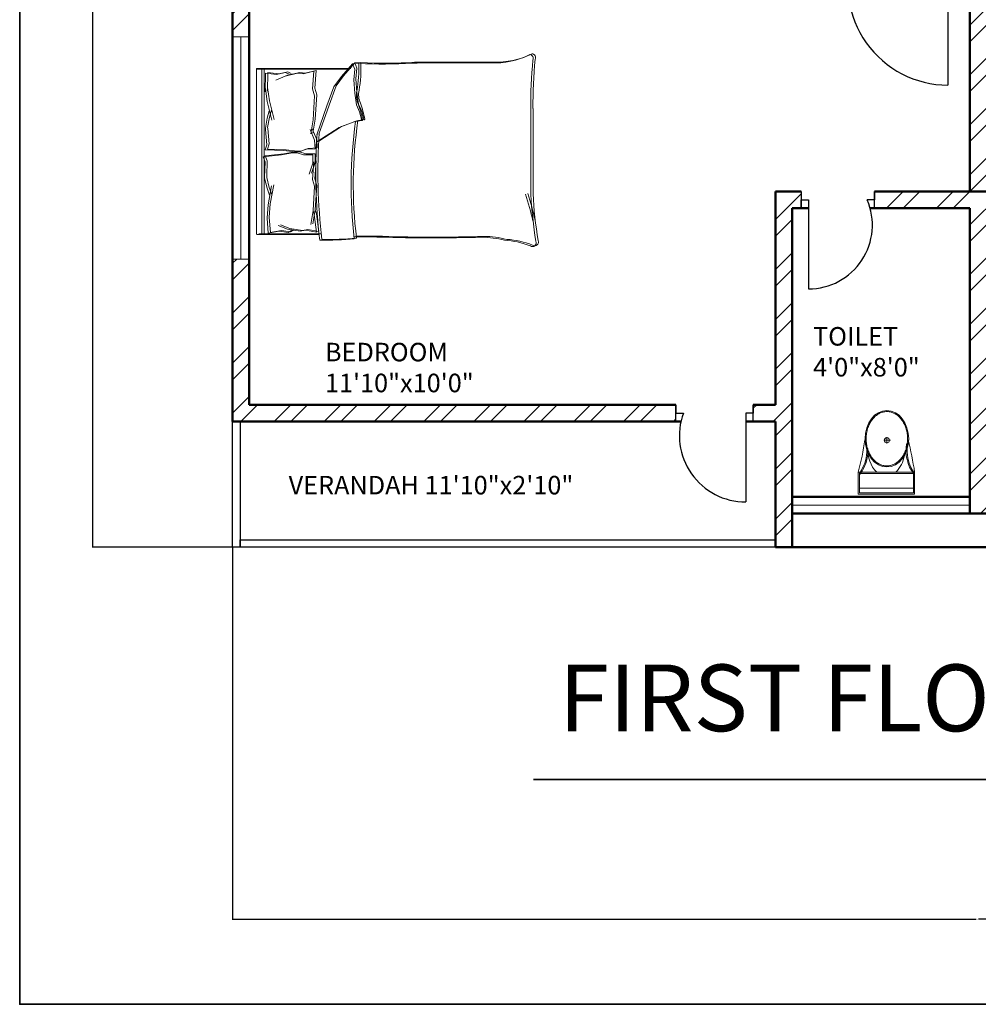
# Model space of a CAD drawing. Units: inches. Extents: x 2129 to 2642, y 1542 to 2414.
# Tile 1 of 9: x 2129 to 2388, y 1542 to 1808. Entities that reach past the tile are written whole.
import ezdxf

# ---------------------------------------------------------------- set-up
doc = ezdxf.new("R2010")
doc.units = ezdxf.units.IN
for name, color, linetype, lineweight in [('A-ANNO-DIMS', 2, 'Continuous', 18), ('A-ANNO-TITL', 7, 'Continuous', 35), ('A-ANNO-TTLB', 7, 'Continuous', 35), ('A-AREA-IDEN', 7, 'Continuous', 18), ('A-DOOR', 3, 'Continuous', 25), ('A-FLOR-FIXT', 9, 'Continuous', 18), ('A-FLOR-RAIL', 80, 'Continuous', 25), ('A-FURN', 8, 'Continuous', 18), ('A-GLAZ', 4, 'Continuous', 18), ('A-WALL', 7, 'Continuous', 50), ('A-WALL-PATT', 252, 'Continuous', 13)]:
    doc.layers.add(name, color=color, linetype=linetype, lineweight=lineweight)
doc.styles.get("Standard").update_dxf_attribs({"font": 'arial.ttf'})
doc.dimstyles.get("Standard").update_dxf_attribs({"dimtxt": 0.18, "dimasz": 0.18, "dimexe": 0.18, "dimexo": 0.0625, "dimgap": 0.09, "dimtad": 0, "dimtih": 1, "dimtoh": 1, "dimdec": 4, "dimzin": 0, "dimdsep": 46, "dimtxsty": 'Standard', "dimcen": 0.09, "dimadec": 0, "dimazin": 0, "dimtfac": 1, "dimtdec": 4, "dimtofl": 0, "dimtmove": 0, "dimatfit": 3, "dimfxl": 1, "dimtolj": 1, "dimtzin": 0, "dimarcsym": 0})

# ---------------------------------------------------------------- blocks, each defined once
blk = doc.blocks.new('A$C31115884')
for p, q in [((283.1, 497.7), (223.4, 497.7)), ((257.5, 466.4), (257.5, 523.2)), ((0, 200), (0, 0)), ((520, 200), (0, 200)), ((10, 190), (10, 10)), ((510, 190), (10, 190)), ((510, 10), (510, 190)), ((520, 0), (520, 200)), ((510, 54.5), (0, 54.5)), ((10, 10), (510, 10)), ((0, 0), (520, 0))]:
    blk.add_line(p, q)
blk.add_circle((255.6, 496.4), 23.6)
for centre, radius, start, end in [((2777.7, -204.6), 2807, 165.4549, 171.71327), ((-294.5, 403.3), 364.7, 324.20913, 9.34987), ((-294.5, 403.3), 374.7, 324.20913, 9.34987), ((805.8, 403.3), 364.7, 170.65013, 215.79087), ((3237, 905), 2807, 188.28673, 194.5451), ((139.5, 406.2), 293.5, 315.84364, 2.65635), ((805.8, 403.3), 374.7, 179.20365, 215.79087), ((383.6, 406.2), 293.5, 190.27735, 224.15636)]:
    blk.add_arc(centre, radius, start, end)
blk.add_ellipse((256.2, 509.9), major_axis=(0, -260.7), ratio=0.772727)
blk.add_open_spline([(256.2, 259.2), (263.1, 259.2), (270, 259.7), (287.8, 262.3), (298.7, 265.1), (319.9, 273.1), (330.2, 278.4), (350.1, 291.1), (359.7, 298.7), (377.7, 315.9), (386.2, 325.5), (401.7, 346.6), (408.8, 358.1), (421.3, 382.5), (426.8, 395.5), (435.9, 422.4), (439.5, 436.4), (444.8, 465.1), (446.5, 479.7), (447.9, 509.2), (447.6, 524), (445, 553.3), (442.7, 567.8), (436.3, 596), (432.1, 609.7), (421.9, 636), (416, 648.6), (402.5, 672.1), (395, 683), (378.6, 703), (369.8, 712.1), (351.1, 728), (341.3, 734.8), (320.9, 746.2), (310.4, 750.7), (288.9, 757.3), (278, 759.4), (256, 761), (245, 760.6), (223.1, 757.2), (212.3, 754.3), (191.1, 746.1), (180.8, 740.7), (160.9, 727.8), (151.4, 720.1), (133.5, 702.7), (125.1, 693), (109.6, 671.7), (102.6, 660.2), (90.2, 635.7), (84.9, 622.7), (76, 595.6), (72.4, 581.6), (67.2, 552.9), (65.6, 538.2), (64.4, 508.8), (64.8, 494), (67.5, 464.7), (69.9, 450.2), (76.6, 422), (80.8, 408.3), (91.1, 382.2), (97.2, 369.7), (110.8, 346.3), (118.4, 335.4), (134.8, 315.6), (143.7, 306.7), (162.4, 290.9), (172.3, 284.2), (192.8, 273), (203.3, 268.6), (224.8, 262.2), (235.8, 260.2), (249.9, 259.3), (253, 259.2), (256.2, 259.2)], degree=3, knots=[0, 0, 0, 0, 0.110105, 0.110105, 0.285049, 0.285049, 0.459994, 0.459994, 0.634938, 0.634938, 0.809882, 0.809882, 0.984827, 0.984827, 1.159771, 1.159771, 1.334715, 1.334715, 1.50966, 1.50966, 1.684604, 1.684604, 1.859549, 1.859549, 2.034493, 2.034493, 2.209437, 2.209437, 2.384382, 2.384382, 2.559326, 2.559326, 2.73427, 2.73427, 2.909215, 2.909215, 3.084159, 3.084159, 3.259103, 3.259103, 3.434048, 3.434048, 3.608992, 3.608992, 3.783936, 3.783936, 3.958881, 3.958881, 4.133825, 4.133825, 4.30877, 4.30877, 4.483714, 4.483714, 4.658658, 4.658658, 4.833603, 4.833603, 5.008547, 5.008547, 5.183491, 5.183491, 5.358436, 5.358436, 5.53338, 5.53338, 5.708324, 5.708324, 5.883269, 5.883269, 6.058213, 6.058213, 6.233158, 6.233158, 6.283185, 6.283185, 6.283185, 6.283185])
blk = doc.blocks.new('BED-DOUBLE')
for p, q in [((3.24, 59.14), (3.24, 76.05)), ((3.24, 74.61), (47.87, 74.61)), ((3.25, 59.14), (3.25, 76.05)), ((3.25, 74.61), (47.87, 74.61)), ((48.08, 76.05), (3.46, 76.05)), ((3.46, 58.54), (3.46, 75.45)), ((3.46, 58.54), (3.46, 75.45)), ((47.87, 76.05), (47.87, 51.2)), ((47.87, 76.05), (47.87, 51.2)), ((48.08, 76.05), (48.08, 75.45)), ((48.08, 75.45), (48.08, 50.6)), ((48.08, 75.45), (48.08, 50.6)), ((3.46, 74.02), (48.08, 74.02)), ((3.46, 74.02), (48.08, 74.02)), ((3.64, 72.93), (7.64, 73.24)), ((3.64, 72.93), (7.64, 73.24)), ((3.64, 72.95), (4.18, 69.98)), ((3.64, 72.95), (4.18, 69.98)), ((3.85, 72.33), (7.85, 72.64)), ((3.85, 72.33), (7.85, 72.64)), ((3.85, 72.35), (4.39, 69.38)), ((3.85, 72.35), (4.39, 69.38)), ((7.64, 73.24), (7.74, 73.22)), ((7.64, 73.24), (7.74, 73.22)), ((7.74, 73.22), (11.31, 72.95)), ((7.74, 73.22), (11.31, 72.95)), ((7.85, 72.64), (7.95, 72.62)), ((7.85, 72.64), (7.95, 72.62)), ((7.95, 72.62), (11.52, 72.35)), ((7.95, 72.62), (11.52, 72.35)), ((11.31, 72.95), (16.44, 72.01)), ((11.31, 72.95), (16.44, 72.01)), ((11.52, 72.35), (16.65, 71.41)), ((11.52, 72.35), (16.65, 71.41)), ((13.87, 72.55), (15.76, 73.22)), ((13.87, 72.55), (15.76, 73.22)), ((14.08, 71.95), (15.97, 72.62)), ((14.08, 71.95), (15.97, 72.62)), ((15.76, 73.22), (18.46, 73.9)), ((15.76, 73.22), (18.46, 73.9)), ((15.97, 72.62), (18.67, 73.3)), ((15.97, 72.62), (18.67, 73.3)), ((18.46, 73.9), (18.76, 73.9)), ((18.46, 73.9), (18.76, 73.9)), ((18.67, 73.3), (18.97, 73.3)), ((18.67, 73.3), (18.97, 73.3)), ((18.76, 73.9), (22.91, 73.76)), ((18.76, 73.9), (22.91, 73.76)), ((18.97, 73.3), (23.12, 73.16)), ((18.97, 73.3), (23.12, 73.16)), ((22.91, 73.76), (24.26, 74.3)), ((22.91, 73.76), (24.26, 74.3)), ((23.12, 73.16), (24.47, 73.7)), ((23.12, 73.16), (24.47, 73.7)), ((24.26, 74.3), (24.8, 69.31)), ((24.26, 74.3), (24.8, 69.31)), ((24.47, 73.7), (25.01, 68.71)), ((24.47, 73.7), (25.01, 68.71)), ((26.12, 73.72), (25.9, 68.7)), ((26.12, 73.72), (25.9, 68.7)), ((26.34, 73.12), (26.11, 68.1)), ((26.34, 73.12), (26.11, 68.1)), ((27.5, 73.27), (26.12, 73.72)), ((27.5, 73.27), (26.12, 73.72)), ((27.72, 72.67), (26.34, 73.12)), ((27.72, 72.67), (26.34, 73.12)), ((31.64, 73.66), (27.5, 73.27)), ((31.64, 73.66), (27.5, 73.27)), ((31.85, 73.06), (27.72, 72.67)), ((31.85, 73.06), (27.72, 72.67)), ((31.94, 73.68), (31.64, 73.66)), ((31.94, 73.68), (31.64, 73.66)), ((32.15, 73.08), (31.85, 73.06)), ((32.15, 73.08), (31.85, 73.06)), ((34.68, 73.17), (31.94, 73.68)), ((34.67, 73.17), (31.94, 73.68)), ((34.89, 72.58), (32.15, 73.08)), ((34.89, 72.58), (32.15, 73.08)), ((39.14, 73.18), (34.08, 71.92)), ((39.14, 73.18), (34.08, 71.92)), ((39.35, 72.58), (34.29, 71.32)), ((39.35, 72.58), (34.29, 71.32)), ((36.6, 72.62), (34.67, 73.17)), ((36.6, 72.62), (34.68, 73.17)), ((36.82, 72.02), (34.89, 72.58)), ((36.82, 72.02), (34.89, 72.58)), ((42.68, 73.67), (39.14, 73.18)), ((42.68, 73.67), (39.14, 73.18)), ((42.9, 73.08), (39.35, 72.58)), ((42.9, 73.08), (39.35, 72.58)), ((46.79, 73.66), (41.75, 73.75)), ((41.75, 73.75), (42.68, 73.67)), ((46.79, 73.66), (41.75, 73.75)), ((41.75, 73.75), (42.68, 73.67)), ((47.01, 73.06), (41.96, 73.15)), ((41.96, 73.15), (42.9, 73.08)), ((47.01, 73.06), (41.96, 73.15)), ((41.96, 73.15), (42.9, 73.08)), ((46.79, 73.66), (46.44, 70.66)), ((46.79, 73.66), (46.44, 70.66)), ((47.01, 73.06), (46.65, 70.06)), ((47.01, 73.06), (46.65, 70.06)), ((4.18, 69.98), (3.77, 67.55)), ((4.18, 69.98), (3.77, 67.55)), ((4.39, 69.38), (3.98, 66.95)), ((4.39, 69.38), (3.99, 66.95)), ((4.72, 67.69), (5.66, 70.25)), ((4.72, 67.69), (5.66, 70.25)), ((4.93, 67.09), (5.87, 69.65)), ((4.93, 67.09), (5.87, 69.65)), ((24.8, 69.31), (25.34, 66.34)), ((24.8, 69.31), (25.34, 66.34)), ((46.04, 68.34), (44.94, 70.84)), ((46.04, 68.34), (44.94, 70.84)), ((46.26, 67.74), (45.15, 70.24)), ((46.26, 67.74), (45.15, 70.24)), ((46.44, 70.66), (46.99, 68.26)), ((46.44, 70.66), (46.99, 68.26)), ((46.65, 70.06), (47.21, 67.66)), ((46.65, 70.06), (47.21, 67.66)), ((3.77, 67.55), (4.31, 66.61)), ((3.77, 67.55), (4.31, 66.61)), ((3.98, 66.95), (4.52, 66.01)), ((3.99, 66.95), (4.53, 66.01)), ((4.18, 64.31), (4.72, 67.69)), ((4.18, 64.31), (4.72, 67.69)), ((4.39, 63.71), (4.93, 67.09)), ((4.39, 63.71), (4.93, 67.09)), ((25.01, 68.71), (25.55, 65.74)), ((25.01, 68.71), (25.55, 65.74)), ((25.9, 68.7), (25.54, 65.7)), ((25.9, 68.7), (25.54, 65.7)), ((26.11, 68.1), (25.76, 65.11)), ((26.11, 68.1), (25.76, 65.11)), ((46.79, 65), (46.04, 68.34)), ((46.79, 65), (46.04, 68.34)), ((47.01, 64.41), (46.26, 67.74)), ((47.01, 64.41), (46.26, 67.74)), ((46.99, 68.26), (46.51, 67.28)), ((46.99, 68.26), (46.51, 67.28)), ((47.21, 67.66), (46.73, 66.69)), ((47.21, 67.66), (46.73, 66.69)), ((4.45, 62.82), (4.18, 64.31)), ((4.45, 62.82), (4.18, 64.31)), ((25.34, 65.12), (24.8, 63.36)), ((25.34, 65.12), (24.8, 63.36)), ((25.55, 64.52), (25.01, 62.77)), ((25.55, 64.52), (25.01, 62.77)), ((25.34, 66.34), (25.34, 65.12)), ((25.34, 66.34), (25.34, 65.12)), ((25.54, 65.7), (25.62, 64.49)), ((25.54, 65.7), (25.62, 64.49)), ((25.55, 65.74), (25.55, 64.52)), ((25.55, 65.74), (25.55, 64.52)), ((25.62, 64.49), (26.27, 62.77)), ((25.62, 64.49), (26.27, 62.77)), ((25.76, 65.11), (25.83, 63.89)), ((25.76, 65.11), (25.83, 63.89)), ((25.83, 63.89), (26.48, 62.18)), ((25.83, 63.89), (26.48, 62.18)), ((46.62, 63.5), (46.79, 65)), ((46.62, 63.5), (46.79, 65)), ((46.83, 62.91), (47.01, 64.41)), ((46.83, 62.91), (47.01, 64.41)), ((3.91, 59.85), (4.45, 62.82)), ((3.91, 59.85), (4.45, 62.82)), ((4.12, 59.26), (4.66, 62.23)), ((4.12, 59.26), (4.66, 62.23)), ((4.66, 62.23), (4.39, 63.71)), ((4.66, 62.23), (4.39, 63.71)), ((5.96, 61.45), (9.72, 60.83)), ((5.96, 61.45), (9.72, 60.83)), ((22.51, 60.86), (19.57, 61.88)), ((22.51, 60.86), (19.57, 61.88)), ((22.72, 60.26), (19.78, 61.28)), ((22.72, 60.26), (19.78, 61.28)), ((24.8, 63.36), (24.8, 60.86)), ((24.8, 63.36), (24.8, 60.86)), ((25.01, 62.77), (25.01, 60.26)), ((25.01, 62.77), (25.01, 60.26)), ((26.27, 62.77), (26.42, 60.27)), ((26.27, 62.77), (26.42, 60.27)), ((26.48, 62.18), (26.64, 59.68)), ((26.48, 62.18), (26.64, 59.68)), ((28.71, 60.42), (31.58, 61.62)), ((28.71, 60.42), (31.58, 61.62)), ((30.41, 61.45), (34.17, 60.83)), ((30.41, 61.45), (34.17, 60.83)), ((47.34, 60.57), (46.62, 63.5)), ((47.34, 60.57), (46.62, 63.5)), ((47.55, 59.98), (46.83, 62.91)), ((47.55, 59.98), (46.83, 62.91)), ((8.67, 60.53), (3.91, 59.85)), ((8.67, 60.53), (3.91, 59.85)), ((8.88, 59.93), (4.12, 59.26)), ((8.88, 59.93), (4.12, 59.26)), ((6.17, 60.86), (9.94, 60.23)), ((6.17, 60.86), (9.94, 60.23)), ((9.72, 60.83), (8.67, 60.53)), ((9.72, 60.83), (8.67, 60.53)), ((9.94, 60.23), (8.88, 59.93)), ((9.94, 60.23), (8.88, 59.93)), ((9.72, 60.83), (16.27, 60.43)), ((9.72, 60.83), (16.27, 60.43)), ((9.94, 60.23), (16.48, 59.83)), ((9.94, 60.23), (16.48, 59.83)), ((16.27, 60.43), (18.1, 60.95)), ((16.27, 60.43), (18.1, 60.95)), ((16.48, 59.83), (18.31, 60.35)), ((16.48, 59.83), (18.31, 60.35)), ((18.1, 60.95), (22.89, 60.57)), ((18.1, 60.95), (22.89, 60.57)), ((18.31, 60.35), (23.11, 59.98)), ((18.31, 60.35), (23.1, 59.98)), ((24.8, 60.86), (22.51, 60.86)), ((24.8, 60.86), (22.51, 60.86)), ((25.01, 60.26), (22.72, 60.26)), ((25.01, 60.26), (22.72, 60.26)), ((26.42, 60.27), (28.71, 60.42)), ((26.42, 60.27), (28.71, 60.42)), ((26.64, 59.68), (28.93, 59.82)), ((26.64, 59.68), (28.93, 59.82)), ((28.25, 59.82), (32.17, 53.75)), ((28.25, 59.82), (32.17, 53.75)), ((28.47, 59.22), (32.38, 53.16)), ((28.47, 59.22), (32.38, 53.16)), ((28.93, 59.82), (31.79, 61.02)), ((28.93, 59.82), (31.79, 61.02)), ((37.95, 57.08), (30.17, 59.82)), ((37.95, 57.08), (30.17, 59.82)), ((38.16, 56.48), (30.38, 59.22)), ((38.16, 56.48), (30.38, 59.22)), ((30.62, 60.86), (34.39, 60.23)), ((30.62, 60.86), (34.38, 60.23)), ((34.17, 60.83), (40.72, 60.43)), ((34.17, 60.83), (40.72, 60.43)), ((34.38, 60.23), (40.93, 59.83)), ((34.39, 60.23), (40.93, 59.83)), ((40.72, 60.43), (42.55, 60.95)), ((40.72, 60.43), (42.55, 60.95)), ((40.93, 59.83), (42.76, 60.35)), ((40.93, 59.83), (42.76, 60.35)), ((42.55, 60.95), (47.34, 60.57)), ((42.55, 60.95), (47.34, 60.57)), ((42.76, 60.35), (47.55, 59.98)), ((42.76, 60.35), (47.55, 59.98)), ((43.16, 55.2), (37.95, 57.08)), ((43.16, 55.2), (37.95, 57.08)), ((43.37, 54.6), (38.16, 56.48)), ((43.37, 54.6), (38.16, 56.48)), ((32.17, 53.75), (33.76, 49.56)), ((32.17, 53.75), (33.76, 49.56)), ((32.38, 53.16), (33.97, 48.96)), ((32.38, 53.16), (33.97, 48.96)), ((45.91, 53.17), (43.16, 55.2)), ((45.91, 53.17), (43.16, 55.2)), ((46.12, 52.58), (43.37, 54.6)), ((46.12, 52.58), (43.37, 54.6)), ((49.37, 50.14), (45.91, 53.17)), ((49.36, 50.14), (45.91, 53.17)), ((49.58, 49.54), (46.12, 52.58)), ((49.58, 49.54), (46.12, 52.58)), ((33.76, 49.56), (34.05, 47.68)), ((33.76, 49.56), (34.05, 47.68)), ((33.97, 48.96), (34.26, 47.09)), ((33.97, 48.96), (34.26, 47.09)), ((34.05, 47.68), (36.36, 48.26)), ((34.05, 47.68), (36.36, 48.26)), ((36.36, 48.26), (38.24, 49.13)), ((36.36, 48.26), (38.24, 49.13)), ((36.57, 47.66), (38.45, 48.53)), ((36.57, 47.66), (38.45, 48.53)), ((38.24, 49.13), (41.42, 49.56)), ((38.24, 49.13), (41.42, 49.56)), ((38.45, 48.53), (41.64, 48.96)), ((38.45, 48.53), (41.64, 48.96)), ((41.42, 49.56), (45.04, 49.85)), ((41.42, 49.56), (45.04, 49.85)), ((41.64, 48.96), (45.25, 49.25)), ((41.64, 48.96), (45.25, 49.25)), ((45.04, 49.85), (47.93, 49.56)), ((45.04, 49.85), (47.93, 49.56)), ((45.25, 49.25), (48.14, 48.96)), ((45.25, 49.25), (48.14, 48.96)), ((47.93, 49.56), (49.37, 50.14)), ((47.93, 49.56), (49.36, 50.14)), ((48.14, 48.96), (49.58, 49.54)), ((48.14, 48.96), (49.58, 49.54)), ((49.44, 48.51), (49.36, 50.14, 3.61)), ((49.44, 48.51), (49.37, 50.14, 3.61)), ((49.65, 47.91), (49.58, 49.54, 3.61)), ((49.65, 47.91), (49.58, 49.54, 3.61)), ((34.26, 47.09), (36.57, 47.66)), ((34.26, 47.09), (36.57, 47.66)), ((14.07, 2.05), (37.05, 2.05)), ((14.07, 2.05), (37.05, 2.05)), ((14.28, 1.46), (37.26, 1.46)), ((14.28, 1.46), (37.26, 1.46))]:
    blk.add_line(p, q)
for centre, radius, start, end in [((79.52, 57.28), 77.79, 178.7218, 185.604), ((79.52, 57.28), 77.79, 178.7218, 185.604), ((19.94, -93.94), 154.04, 86.0865, 96.7821), ((19.94, -93.94), 154.04, 86.0865, 96.7821), ((20.16, -94.54), 154.04, 86.0865, 96.7821), ((20.16, -94.54), 154.04, 86.0865, 96.7821), ((79.73, 56.69), 77.79, 178.7218, 185.604), ((79.73, 56.69), 77.79, 178.7218, 185.604), ((16.58, -69.91), 120.47, 81.7845, 96.9006), ((16.58, -69.91), 120.47, 81.7845, 96.9006), ((16.79, -70.51), 120.47, 81.7845, 96.9006), ((16.79, -70.51), 120.47, 81.7845, 96.9006), ((-156.22, 46.94), 158.84, 358.4762, 1.0082), ((-156.22, 46.94), 158.84, 358.4762, 1.0082), ((-156.01, 46.34), 158.84, 358.4762, 1.0082), ((-156.01, 46.34), 158.84, 358.4762, 1.0082), ((29.09, 74.66), 27.69, 280.6617, 289.8806), ((29.09, 74.66), 27.69, 280.6617, 289.8806), ((29.3, 74.07), 27.69, 280.6617, 289.8806), ((29.3, 74.07), 27.69, 280.6617, 289.8806), ((40.85, 43.3), 5.81, 78.6608, 113.7384), ((40.85, 43.3), 5.81, 78.6608, 113.7384), ((41.06, 42.71), 5.81, 78.6608, 113.7384), ((41.06, 42.71), 5.81, 78.6608, 113.7384), ((47.93, 82.26), 33.79, 259.8763, 272.5657), ((47.93, 82.26), 33.79, 259.8763, 272.5657), ((48.14, 81.67), 33.79, 259.8763, 272.5657), ((48.14, 81.67), 33.79, 259.8763, 272.5657), ((170.19, 42.14), 120.92, 176.9791, 183.8365), ((170.19, 42.14), 120.92, 176.9791, 183.8365), ((170.4, 41.54), 120.92, 176.9791, 183.8365), ((170.4, 41.54), 120.92, 176.9791, 183.8365), ((34.21, 47.62), 0.172, 160.2464, 271.1377), ((34.21, 47.62), 0.172, 160.2464, 271.1377), ((34.42, 47.03), 0.172, 160.2464, 271.1377), ((34.42, 47.03), 0.172, 160.2464, 271.1377), ((452.7, 28.79), 450.36, 178.2277, 181.7185), ((452.7, 28.79), 450.36, 178.2277, 181.7185), ((452.91, 28.19), 450.36, 178.2277, 181.7185), ((452.91, 28.19), 450.36, 178.2277, 181.7185), ((-4210.02, 12.72), 4259.62, 0.00217, 0.28689), ((-4210.02, 12.72), 4259.62, 0.00217, 0.28689), ((-4209.81, 12.12), 4259.62, 0.00217, 0.28689), ((-4209.81, 12.12), 4259.62, 0.00217, 0.28689), ((-25.12, 15.81), 27.67, 346.0648, 358.9113), ((-25.12, 15.81), 27.67, 346.0648, 358.9113), ((-24.9, 15.21), 27.67, 346.0648, 358.9113), ((-24.9, 15.21), 27.67, 346.0648, 358.9113), ((71.11, 11.93), 21.54, 177.4714, 206.4681), ((71.11, 11.93), 21.54, 177.4714, 206.4681), ((71.33, 11.33), 21.54, 177.4714, 206.4681), ((71.32, 11.33), 21.54, 177.4714, 206.4681), ((-20.22, 10.43), 22, 337.9751, 356.652), ((-20.22, 10.43), 22, 337.9751, 356.652), ((-20.01, 9.83), 22, 337.9751, 356.652), ((-20.01, 9.83), 22, 337.9751, 356.652), ((-16.08, 98.19), 99.41, 283.3832, 287.7053), ((-16.08, 98.19), 99.41, 283.3832, 287.7053), ((-15.87, 97.59), 99.41, 283.3832, 287.7053), ((-15.87, 97.59), 99.41, 283.3832, 287.7053), ((1.02, 1.61), 1.02, 146.1736, 293.4781), ((1.02, 1.61), 1.02, 146.1736, 293.4781), ((1.23, 1.01), 1.02, 146.1736, 293.4781), ((1.23, 1.01), 1.02, 146.1736, 293.4781), ((20.01, -111.48), 113.69, 92.9958, 99.4091), ((20.01, -111.48), 113.69, 92.9958, 99.4091), ((20.22, -112.08), 113.69, 92.9958, 99.4091), ((20.22, -112.08), 113.69, 92.9958, 99.4091), ((38.43, -122.17), 124.23, 84.4998, 90.6351), ((38.43, -122.17), 124.23, 84.4998, 90.6351), ((38.64, -122.76), 124.23, 84.4998, 90.6351), ((38.64, -122.76), 124.23, 84.4998, 90.6351), ((50.81, 2.4), 1.03, 242.6588, 356.02), ((50.81, 2.4), 1.03, 242.6588, 356.02), ((51.02, 1.81), 1.03, 242.6588, 356.02), ((51.02, 1.81), 1.03, 242.6588, 356.02)]:
    blk.add_arc(centre, radius, start, end)
blk = doc.blocks.new('WIN-60-B')
for p, q in [((4.5, 60), (0, 60)), ((0, 60), (2.25, 60)), ((2.25, 60), (2.25, 0)), ((2.25, 0), (0, 0)), ((0, 0), (4.5, 0))]:
    blk.add_line(p, q)
blk = doc.blocks.new('*D34')
at = {"layer": 'A-ANNO-DIMS', "color": 0, "lineweight": -2, "transparency": 16777216}
for p, q in [((2186.9, 1665.66), (2186.9, 1565.16)), ((2588.9, 1665.66), (2588.9, 1565.16)), ((2187.08, 1565.34), (2387.61, 1565.34)), ((2588.72, 1565.34), (2388.2, 1565.34))]:
    blk.add_line(p, q, dxfattribs=at)
at = {"layer": 'A-ANNO-DIMS', "color": 0, "transparency": 16777216}
for points in [[(2187.08, 1565.37), (2187.08, 1565.31), (2186.9, 1565.34)], [(2588.72, 1565.37), (2588.72, 1565.31), (2588.9, 1565.34)]]:
    blk.add_solid(points, dxfattribs=at)
at = {"layer": 'Defpoints', "color": 0, "transparency": 16777216}
for p in [(2186.9, 1665.72), (2588.9, 1665.72), (2588.9, 1565.34)]:
    blk.add_point(p, dxfattribs=at)
at = {"layer": 'A-ANNO-DIMS', "color": 0, "transparency": 16777216, "insert": (2387.9, 1565.34), "char_height": 0.18, "attachment_point": 5}
blk.add_mtext('\\A1;402', dxfattribs=at)
blk = doc.blocks.new('*D35')
at = {"layer": 'A-ANNO-DIMS', "color": 0, "lineweight": -2, "transparency": 16777216}
for p, q in [((2186.84, 2340.22), (2148.97, 2340.22)), ((2149.15, 2340.04), (2149.15, 2003.15)), ((2149.15, 1665.9), (2149.15, 2002.79)), ((2186.84, 1665.72), (2148.97, 1665.72))]:
    blk.add_line(p, q, dxfattribs=at)
at = {"layer": 'A-ANNO-DIMS', "color": 0, "transparency": 16777216}
for points in [[(2149.12, 2340.04), (2149.18, 2340.04), (2149.15, 2340.22)], [(2149.12, 1665.9), (2149.18, 1665.9), (2149.15, 1665.72)]]:
    blk.add_solid(points, dxfattribs=at)
at = {"layer": 'Defpoints', "color": 0, "transparency": 16777216}
for p in [(2149.15, 2340.22), (2186.9, 2340.22), (2186.9, 1665.72)]:
    blk.add_point(p, dxfattribs=at)
at = {"layer": 'A-ANNO-DIMS', "color": 0, "transparency": 16777216, "insert": (2149.15, 2002.97), "char_height": 0.18, "attachment_point": 5}
blk.add_mtext('\\A1;674.5', dxfattribs=at)

msp = doc.modelspace()

# ---------------------------------------------------------------- hatches: boundary and pattern name
at = {"layer": 'A-WALL-PATT'}
h = msp.add_hatch(dxfattribs=at)
h.set_pattern_fill('ANSI32', color=256)
h.paths.add_polyline_path([(2306.2606, 2305.9717), (2306.2606, 2308.2217), (2276.3515, 2308.2217), (2276.3515, 2303.7217), (2306.2606, 2303.7217)])
h.paths.add_polyline_path([(2216.3515, 2305.9717), (2216.3515, 2308.2217), (2186.9043, 2308.2217), (2186.9043, 2278.1696), (2191.4043, 2278.1696), (2191.4043, 2303.7217), (2216.3515, 2303.7217)])
h.paths.add_polyline_path([(2339.9043, 2335.7217), (2362.1938, 2335.7217), (2362.1938, 2340.2217), (2335.4043, 2340.2217), (2335.4043, 2308.2217), (2329.3487, 2308.2217), (2329.3487, 2305.9717), (2329.3487, 2303.7217), (2335.4043, 2303.7217), (2335.4043, 2186.7217), (2329.4345, 2186.7217), (2329.4345, 2182.2217), (2335.4043, 2182.2217), (2335.4043, 2174.7178), (2339.9043, 2174.7178), (2339.9043, 2182.2217), (2339.9043, 2303.7217)])
h.paths.add_polyline_path([(2440.4043, 2340.2217), (2411.654, 2340.2217), (2411.654, 2335.7217), (2435.9043, 2335.7217), (2435.9043, 2303.7217), (2435.9043, 2182.2217), (2435.9043, 2174.1935), (2438.1543, 2174.1935), (2440.4043, 2174.1935), (2440.4043, 2182.2217), (2444.653, 2182.2217), (2444.653, 2184.4717), (2444.653, 2186.7217), (2440.4043, 2186.7217), (2440.4043, 2303.7217), (2445.8547, 2303.7217), (2445.8547, 2308.2217), (2440.4043, 2308.2217)])
h.paths.add_polyline_path([(2498.2381, 2308.2217), (2470.3901, 2308.2217), (2470.3901, 2303.7217), (2498.2381, 2303.7217), (2498.2381, 2305.9717)])
h.paths.add_polyline_path([(2588.9043, 2308.2217), (2586.9043, 2308.2217), (2558.2381, 2308.2217), (2558.2381, 2303.7217), (2584.4043, 2303.7217), (2584.4043, 2279.1087), (2588.9043, 2279.1087)])
h.paths.add_polyline_path([(2588.9043, 2219.1087), (2584.4043, 2219.1087), (2584.4043, 2186.7217), (2478.0667, 2186.7217), (2478.0667, 2182.2217), (2584.4043, 2182.2217), (2584.4043, 2157.7883), (2588.9043, 2157.7883)])
h.paths.add_polyline_path([(2588.9043, 2097.7883), (2584.6063, 2097.7883), (2584.6063, 2075.5462, -0.09241561), (2584.4043, 2074.4627), (2584.4043, 2064.2217), (2495.9043, 2064.2217), (2495.9043, 2040.4611), (2500.4043, 2040.4611), (2500.4043, 2059.7217), (2584.4043, 2059.7217), (2584.4043, 2052.2164), (2588.9043, 2052.2164)])
h.paths.add_polyline_path([(2588.9043, 2028.2164), (2584.4043, 2028.2164), (2584.4043, 2011.7217), (2500.4043, 2011.7217), (2500.4043, 2015.243), (2498.1543, 2015.243), (2495.9043, 2015.243), (2495.9043, 2007.2217), (2495.9043, 2003.7597), (2500.4043, 2003.7597), (2500.4043, 2007.2217), (2584.4043, 2007.2217), (2584.4043, 1992.1997), (2588.9043, 1992.1997)])
h.paths.add_polyline_path([(2588.9043, 1956.1997), (2584.4043, 1956.1997), (2584.4043, 1941.2217), (2500.4043, 1941.2217), (2500.4043, 1985.1493), (2498.1543, 1985.1493), (2495.9043, 1985.1493), (2495.9043, 1941.2217), (2435.9043, 1941.2217), (2435.9043, 1930.3963), (2440.4043, 1930.3963), (2440.4043, 1936.7217), (2584.4043, 1936.7217), (2584.4043, 1909.8406), (2588.9043, 1909.8406)])
h.paths.add_polyline_path([(2588.9043, 1849.8406), (2584.4043, 1849.8406), (2584.4043, 1801.3526), (2588.9043, 1801.3526)])
h.paths.add_polyline_path([(2584.4043, 1828.7217), (2495.9043, 1828.7217), (2440.4043, 1828.7217), (2440.4043, 1905.2159), (2438.1543, 1905.2159), (2435.9043, 1905.2159), (2435.9043, 1828.7217), (2428.9101, 1828.7217), (2428.9101, 1824.2217), (2584.4043, 1824.2217)])
h.paths.add_polyline_path([(2588.9043, 1741.3526), (2584.4043, 1741.3526), (2584.4043, 1704.2217), (2468.3173, 1704.2217), (2468.3173, 1701.9717), (2468.3173, 1699.7217), (2588.9043, 1699.7217)])
h.paths.add_polyline_path([(2442.4043, 1761.7217), (2435.0216, 1761.7217), (2435.0216, 1757.2217), (2437.9043, 1757.2217), (2437.9043, 1665.7217), (2442.4043, 1665.7217), (2442.4043, 1667.7217), (2442.4043, 1699.7217), (2446.6907, 1699.7217), (2446.6907, 1701.9717), (2446.6907, 1704.2217), (2442.4043, 1704.2217)])
h.paths.add_polyline_path([(2390.4043, 1757.2217), (2410.8996, 1757.2217), (2410.8996, 1761.7217), (2360.1741, 1761.7217), (2360.1741, 1759.4717), (2360.1741, 1757.2217), (2385.9043, 1757.2217), (2385.9043, 1674.8326), (2390.4043, 1674.8326)])
h.paths.add_polyline_path([(2337.9043, 1757.2217), (2340.3592, 1757.2217), (2340.3592, 1759.4717), (2340.3592, 1761.7217), (2333.4043, 1761.7217), (2333.4043, 1704.2217), (2327.381, 1704.2217), (2327.381, 1701.9717), (2327.381, 1699.7217), (2333.4043, 1699.7217), (2333.4043, 1665.7217), (2337.9043, 1665.7217)])
h.paths.add_polyline_path([(2191.4043, 1743.4804), (2186.9043, 1743.4804), (2186.9043, 1699.7217), (2188.9043, 1699.7217), (2191.4043, 1699.7217), (2306.5617, 1699.7217), (2306.5617, 1704.2217), (2191.4043, 1704.2217)])
h.paths.add_polyline_path([(2191.4043, 1859.8992), (2186.9043, 1859.8992), (2186.9043, 1803.4804), (2189.1543, 1803.4804), (2191.4043, 1803.4804)])
h.paths.add_polyline_path([(2352.5445, 1828.7217), (2191.4043, 1828.7217), (2191.4043, 1824.2217), (2333.4043, 1824.2217), (2352.5445, 1824.2217), (2352.5445, 1826.4717)])
h.paths.add_polyline_path([(2390.4043, 2085.328), (2385.9043, 2085.328), (2385.9043, 1828.7217), (2381.9668, 1828.7217), (2381.9668, 1826.4717), (2381.9668, 1824.2217), (2385.9043, 1824.2217), (2385.9043, 1761.7217), (2390.4043, 1761.7217), (2390.4043, 1824.2217), (2394.1868, 1824.2217), (2394.1868, 1827.6339), (2394.1868, 1828.7217), (2390.4043, 1828.7217)])
h.paths.add_polyline_path([(2339.9043, 1941.2217), (2335.4043, 1941.2217), (2279.9043, 1941.2217), (2279.9043, 1981.3432), (2277.6543, 1981.3432), (2275.4043, 1981.3432), (2275.4043, 1941.2217), (2191.4043, 1941.2217), (2191.4043, 1958.1079), (2186.9043, 1958.1079), (2186.9043, 1919.8992), (2189.1543, 1919.8992), (2191.4043, 1919.8992), (2191.4043, 1936.7217), (2279.9043, 1936.7217), (2335.4043, 1936.7217), (2335.4043, 1931.1382), (2339.9043, 1931.1382)])
h.paths.add_polyline_path([(2339.9043, 1902.7544), (2337.6543, 1902.7544), (2335.4043, 1902.7544), (2335.4043, 1828.7217), (2339.9043, 1828.7217)])
h.paths.add_polyline_path([(2279.9043, 2015.263), (2277.6543, 2015.263), (2275.4043, 2015.263), (2275.4043, 2011.7217), (2191.4043, 2011.7217), (2191.4043, 2026.6781), (2186.9043, 2026.6781), (2186.9043, 1994.1079), (2189.1543, 1994.1079), (2191.4043, 1994.1079), (2191.4043, 2007.2217), (2275.4043, 2007.2217), (2275.4043, 2003.2288), (2279.9043, 2003.2288), (2279.9043, 2007.2217)])
h.paths.add_polyline_path([(2296.0216, 2186.7217), (2191.4043, 2186.7217), (2191.4043, 2218.1696), (2186.9043, 2218.1696), (2186.9043, 2158.4509), (2191.4043, 2158.4509), (2191.4043, 2182.2217), (2296.0216, 2182.2217), (2296.0216, 2184.4717)])
h.paths.add_polyline_path([(2191.4043, 2098.4509), (2189.1543, 2098.4509), (2186.9043, 2098.4509), (2186.9043, 2050.6781), (2189.0487, 2050.6781), (2191.4043, 2050.6781), (2191.4043, 2059.7217), (2275.4043, 2059.7217), (2275.4043, 2038.4133), (2279.9043, 2038.4133), (2279.9043, 2064.2217), (2191.4043, 2064.2217)])
h.paths.add_polyline_path([(2268.3923, 1605.9386), (2516.3159, 1605.9386), (2516.3159, 1643.0314), (2268.3923, 1643.0314)], flags=9)
h.paths.add_polyline_path([(2399.6079, 1710.4489), (2428.8405, 1710.4489), (2428.8405, 1729.1062), (2399.6079, 1729.1062)], flags=9)
h.paths.add_polyline_path([(2342.1483, 1708.9956), (2371.3809, 1708.9956), (2371.3809, 1727.653), (2342.1483, 1727.653)], flags=9)
h.paths.add_polyline_path([(2200.7404, 1677.2519), (2282.3059, 1677.2519), (2282.3059, 1687.5555), (2200.7404, 1687.5555)], flags=9)
h.paths.add_polyline_path([(2209.8153, 1704.7448), (2250.627, 1704.7448), (2250.627, 1723.4021), (2209.8153, 1723.4021)], flags=25)
h.paths.add_polyline_path([(2213.9996, 1911.284), (2252.84, 1911.284), (2252.84, 1929.9413), (2213.9996, 1929.9413)], flags=9)
h.paths.add_polyline_path([(2210.8865, 1962.0987), (2244.0447, 1962.0987), (2244.0447, 1980.7561), (2210.8865, 1980.7561)], flags=25)
h.paths.add_polyline_path([(2219.0745, 2037.6131), (2248.2321, 2037.6131), (2248.2321, 2056.2705), (2219.0745, 2056.2705)], flags=9)
h.paths.add_polyline_path([(2379.9702, 2099.0686), (2409.3767, 2099.0686), (2409.3767, 2117.7259), (2379.9702, 2117.7259)], flags=9)
h.paths.add_polyline_path([(2375.9312, 2160.3752), (2405.3173, 2160.3752), (2405.3173, 2179.0325), (2375.9312, 2179.0325)], flags=9)
h.paths.add_polyline_path([(2269.5058, 2112.1824), (2310.3175, 2112.1824), (2310.3175, 2130.8397), (2269.5058, 2130.8397)], flags=9)
h.paths.add_polyline_path([(2209.6567, 2193.667), (2248.4971, 2193.667), (2248.4971, 2212.3243), (2209.6567, 2212.3243)], flags=25)
h.paths.add_polyline_path([(2491.6289, 1675.447), (2573.1944, 1675.447), (2573.1944, 1685.7506), (2491.6289, 1685.7506)], flags=9)
h.paths.add_polyline_path([(2492.0585, 1710.4489), (2530.8989, 1710.4489), (2530.8989, 1729.1062), (2492.0585, 1729.1062)], flags=25)
h.paths.add_polyline_path([(2495.6634, 1908.8646), (2534.5038, 1908.8646), (2534.5038, 1927.522), (2495.6634, 1927.522)], flags=9)
h.paths.add_polyline_path([(2516.7779, 1955.9942), (2549.9362, 1955.9942), (2549.9362, 1974.6516), (2516.7779, 1974.6516)], flags=25)
h.paths.add_polyline_path([(2509.7444, 2034.6896), (2538.902, 2034.6896), (2538.902, 2053.347), (2509.7444, 2053.347)], flags=9)
h.paths.add_polyline_path([(2467.8454, 2111.9593), (2508.6571, 2111.9593), (2508.6571, 2130.6167), (2467.8454, 2130.6167)], flags=9)
h.paths.add_polyline_path([(2528.5267, 2189.1742), (2567.3671, 2189.1742), (2567.3671, 2207.8316), (2528.5267, 2207.8316)], flags=25)
h.paths.add_polyline_path([(2483.7603, 2319.9841), (2557.5563, 2319.9841), (2557.5563, 2330.2877), (2483.7603, 2330.2877)], flags=9)
h.paths.add_polyline_path([(2204.078, 2317.0445), (2277.874, 2317.0445), (2277.874, 2327.3481), (2204.078, 2327.3481)], flags=9)

# ---------------------------------------------------------------- linework, layer by layer
at = {"layer": 'A-ANNO-TITL'}
msp.add_line((2268.1427, 1603.0854), (2517.3006, 1603.0854), dxfattribs=at)
at = {"layer": 'A-ANNO-TTLB'}
msp.add_lwpolyline([(2129.4387, 2413.7704), (2642.2731, 2413.7704), (2642.2731, 1542.3836), (2129.4387, 1542.3836)], close=True, dxfattribs=at)
at = {"layer": 'A-DOOR'}
for p, q in [((2379.9668, 1826.4717), (2379.9668, 1790.4717)), ((2340.3592, 1761.7217), (2340.3592, 1757.2217)), ((2340.3592, 1757.2217), (2340.3592, 1759.4717)), ((2340.3592, 1759.4717), (2342.3592, 1759.4717)), ((2342.3592, 1759.4717), (2342.3592, 1735.4717)), ((2360.1741, 1759.4717), (2358.1741, 1759.4717)), ((2360.1741, 1757.2217), (2360.1741, 1761.7217)), ((2360.1741, 1761.7217), (2360.1741, 1759.4717)), ((2306.5617, 1699.7217), (2306.5617, 1704.2217)), ((2306.5617, 1704.2217), (2306.5617, 1701.9717)), ((2327.381, 1699.7217), (2327.381, 1704.2217)), ((2327.381, 1704.2217), (2327.381, 1701.9717)), ((2306.5617, 1701.9717), (2308.5617, 1701.9717)), ((2327.381, 1701.9717), (2325.381, 1701.9717)), ((2325.381, 1701.9717), (2325.381, 1677.9717)), ((2327.381, 1701.9717), (2327.381, 1701.9717))]:
    msp.add_line(p, q, dxfattribs=at)
for centre, radius, start, end in [((2379.9668, 1817.448), 26.9763, 160.457565, 270), ((2342.3592, 1752.6823), 17.2106, 270, 23.233888), ((2325.381, 1695.8652), 17.8935, 160.045854, 270)]:
    msp.add_arc(centre, radius, start, end, dxfattribs=at)
at = {"layer": 'A-FLOR-RAIL'}
for p, q in [((2186.9043, 1665.7217), (2186.9043, 1699.7217)), ((2188.9043, 1699.7217), (2188.9043, 1665.7217)), ((2188.9043, 1665.7217), (2188.9043, 1667.7217)), ((2188.9043, 1667.7217), (2333.4043, 1667.7217)), ((2333.4043, 1665.7217), (2333.4043, 1667.7217)), ((2333.4043, 1665.7217), (2186.9043, 1665.7217))]:
    msp.add_line(p, q, dxfattribs=at)
at = {"layer": 'A-GLAZ'}
msp.add_line((2337.9043, 1677.0587), (2385.9043, 1677.0587), dxfattribs=at)
at = {"layer": 'A-WALL'}
for p, q in [((2186.9043, 2308.2217), (2186.9043, 1699.7217)), ((2191.4043, 1936.7217), (2191.4043, 1704.2217)), ((2385.9043, 1824.2217), (2385.9043, 1761.7217)), ((2333.4043, 1761.7217), (2333.4043, 1704.2217)), ((2333.4043, 1761.7217), (2333.4043, 1757.2217)), ((2340.3592, 1761.7217), (2333.4043, 1761.7217)), ((2410.8996, 1761.7217), (2360.1741, 1761.7217)), ((2337.9043, 1757.2217), (2342.3592, 1757.2217)), ((2337.9043, 1665.7217), (2337.9043, 1757.2217)), ((2358.9604, 1757.2217), (2385.9043, 1757.2217)), ((2385.9043, 1674.8326), (2385.9043, 1757.2217)), ((2306.5617, 1704.2217), (2191.4043, 1704.2217)), ((2333.4043, 1704.2217), (2327.381, 1704.2217)), ((2191.4043, 1699.7217), (2186.9043, 1699.7217)), ((2191.4043, 1699.7217), (2307.908, 1699.7217)), ((2325.381, 1699.7217), (2333.4043, 1699.7217)), ((2333.4043, 1699.7217), (2333.4043, 1665.7217)), ((2337.9043, 1665.7217), (2337.9043, 1699.7217)), ((2385.9043, 1679.3326), (2337.9043, 1679.3326)), ((2337.9043, 1674.8326), (2437.9043, 1674.8326)), ((2333.4043, 1665.7217), (2442.4043, 1665.7217))]:
    msp.add_line(p, q, dxfattribs=at)

# ---------------------------------------------------------------- block references
at = {"layer": 'A-FLOR-FIXT', "xscale": -0.0292470664339069, "yscale": 0.0292470664339069, "zscale": 0.0292470664339069}
msp.add_blockref('A$C31115884', (2370.9685, 1680.1141), dxfattribs=at)
at = {"layer": 'A-FURN', "rotation": 89.99999983318563}
msp.add_blockref('BED-DOUBLE', (2269.4327, 1746.8864), dxfattribs=at)
msp.add_blockref('BED-DOUBLE', (2269.4327, 1746.8864), dxfattribs=at)
at = {"layer": 'A-GLAZ'}
msp.add_blockref('WIN-60-B', (2186.904, 1743.48), dxfattribs=at)

# ---------------------------------------------------------------- texts
at = {"layer": 'A-ANNO-TITL', "insert": (2274.9551, 1634.0867), "char_height": 18, "attachment_point": 1}
msp.add_mtext_dynamic_manual_height_columns('FIRST FLOOR PLAN ', width=400.560432, gutter_width=12.5, heights=[0], dxfattribs=at)
at = {"layer": 'A-AREA-IDEN', "char_height": 5, "attachment_point": 1}
for s, width, insert in [('TOILET\\P4\'0"x8\'0"', 67.542922, (2343.562, 1725.1683)), ('BEDROOM\\P11\'10"x10\'0"', 151.240485, (2211.8258, 1720.9175)), ('VERANDAH 11\'10"x2\'10"', 135.883253, (2202.0211, 1685.0026))]:
    msp.add_mtext_dynamic_manual_height_columns(s, width=width, gutter_width=12.5, heights=[0], dxfattribs=dict(at, insert=insert))

# ---------------------------------------------------------------- dimensions: what is measured, and where the dimension line sits
at = {"layer": 'A-ANNO-DIMS'}
dim = msp.add_linear_dim(base=(2149.1543, 2340.2217), p1=(2186.9043, 1665.7217), p2=(2186.9043, 2340.2217), angle=90, dimstyle='Standard', override={"dimdec": 1, "dimlfac": 1, "dimrnd": 0, "dimzin": 0, "dimdsep": 46, "dimlunit": 2}, dxfattribs=at)
dim.commit()
dim.dimension.update_dxf_attribs({"geometry": '*D35', "text_midpoint": (2149.1543, 2002.9717)})
dim = msp.add_linear_dim(base=(2588.9043, 1565.3354), p1=(2186.9043, 1665.7217), p2=(2588.9043, 1665.7217), dimstyle='Standard', override={"dimdec": 0, "dimlfac": 1, "dimrnd": 0, "dimzin": 0, "dimdsep": 46, "dimlunit": 2}, dxfattribs=at)
dim.commit()
dim.dimension.update_dxf_attribs({"geometry": '*D34', "text_midpoint": (2387.9043, 1565.3354)})

doc.saveas('drawing.dxf')
